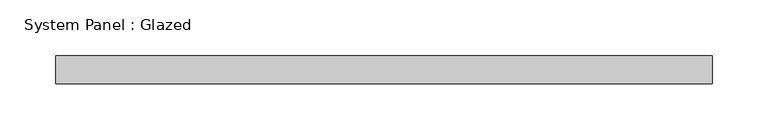
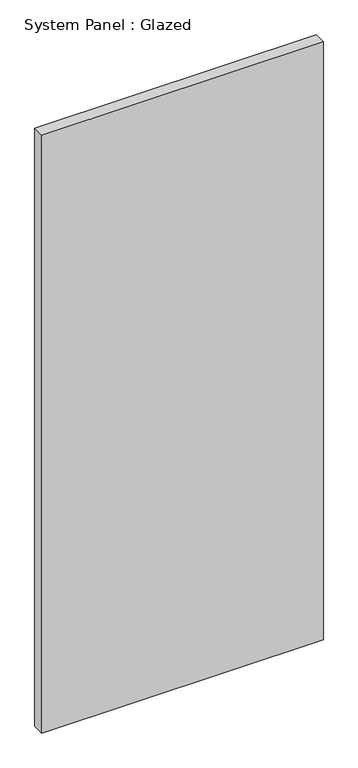
"""IFC4 building model written with IfcOpenShell, lengths in millimetres: plate geometry, System Panel : Glazed."""

from ifc_helpers import new_model, si_unit, origin, origin_with_axes, place, context, project, spatial, polyline, outline, extrude, source, transform, mapped, element, save


def system_panel_glazed_06506daa(model_context):
    return source(origin(), model_context, "Body", "SweptSolid", [
        extrude(outline(polyline([(295.275, 19.05), (-295.275, 19.05), (-295.275, 44.45), (295.275, 44.45), (295.275, 19.05)])), origin_with_axes(), (0.0, 0.0, 1.0), 1325.5193485),
    ])


if __name__ == "__main__":
    model = new_model("IFC4")
    model_context = context("Model", 3, world=origin())
    ifc_project = project(units=[si_unit("LENGTHUNIT", "METRE", prefix="MILLI")], contexts=[model_context])
    site = spatial("IfcSite", under=ifc_project)
    building = spatial("IfcBuilding", under=site)
    placement = place(None, origin())
    system_panel_glazed_shape = system_panel_glazed_06506daa(model_context)
    element("IfcPlate", 1, ObjectType="System Panel : Glazed", at=placement, inside=building, context=model_context, shape_type="MappedRepresentation", body=[
        mapped(system_panel_glazed_shape, transform((0.0, 0.0, 0.0), x_axis=(1.0, 0.0, 0.0), y_axis=(0.0, 1.0, 0.0), z_axis=(0.0, 0.0, 1.0))),
    ])
    save(model, "model.ifc")

# Revit data of these elements
# Type "System Panel : Glazed"
#   Construction Type Id = "GSP4R"
#   Analytic Construction = "1/8 in Pilkington single glazing"
#   Visual Light Transmittance = 0.9
#   Solar Heat Gain Coefficient = 0.86
#   Heat Transfer Coefficient (U) = 1.18115 BTU/(h·ft²·°F)
#   Define Thermal Properties by = 1
# Element 1 (IfcPlate, "System Panel : Glazed")
#   Materials on its faces: "Glass"
# Materials
#   "Glass": class "Glass", colour RGB 0 128 192, transparency 0.75, Description = "Soda Lime Glass", Cost = 0
